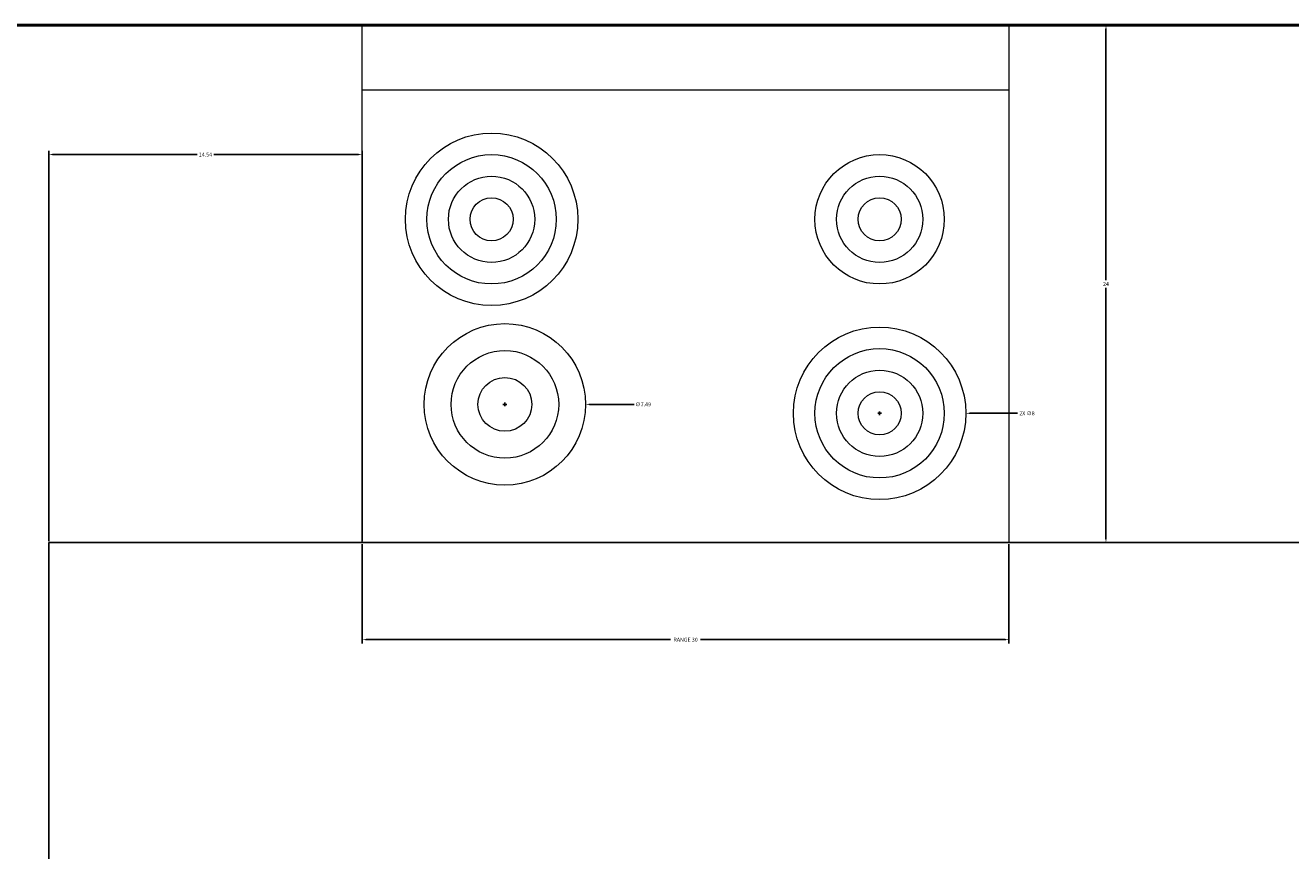
# Model space of a CAD drawing. Units: inches. Extents: x 2621 to 2849, y 2066 to 2463.
# Tile 10 of 28: x 2671 to 2729, y 2277 to 2315. Entities that reach past the tile are written whole.
import ezdxf

# ---------------------------------------------------------------- set-up
doc = ezdxf.new("R2010")
doc.units = ezdxf.units.IN
for name, color, linetype, lineweight in [('A-ANNO-DIMS', 2, 'Continuous', 18), ('A-EQPM', 8, 'Continuous', 18), ('A-FLOR-CASE', 9, 'Continuous', 25), ('A-WALL', 7, 'Continuous', 50)]:
    doc.layers.add(name, color=color, linetype=linetype, lineweight=lineweight)
doc.styles.get("Standard").update_dxf_attribs({"font": 'arial.ttf'})
doc.dimstyles.get("Standard").update_dxf_attribs({"dimtxt": 0.18, "dimasz": 0.18, "dimexe": 0.18, "dimexo": 0.0625, "dimgap": 0.09, "dimtad": 0, "dimtih": 1, "dimtoh": 1, "dimdec": 4, "dimzin": 0, "dimdsep": 46, "dimtxsty": 'Standard', "dimcen": 0.09, "dimadec": 0, "dimazin": 0, "dimtfac": 1, "dimtdec": 4, "dimtofl": 0, "dimtmove": 0, "dimatfit": 3, "dimfxl": 1, "dimtolj": 1, "dimtzin": 0, "dimarcsym": 0})

# ---------------------------------------------------------------- blocks, each defined once
blk = doc.blocks.new('Range-Oven - 30 in top')
blk.add_line((0, -3), (30, -3))
blk.add_lwpolyline([(0, -24), (0, 0), (30, 0), (30, -24)], close=True)
for centre, radius in [((6, -9), 4), ((6, -9), 3), ((24, -9), 3), ((6, -9), 2), ((24, -9), 2), ((6, -9), 1), ((24, -9), 1), ((6.618, -17.584), 3.745), ((24, -18), 4), ((6.618, -17.584), 2.496), ((24, -18), 3), ((6.618, -17.584), 1.248), ((24, -18), 2), ((24, -18), 1)]:
    blk.add_circle(centre, radius)
blk = doc.blocks.new('*D21')
at = {"layer": 'A-ANNO-DIMS', "color": 0, "lineweight": -2, "transparency": 16777216}
for p, q in [((2686.41, 2291.312), (2686.41, 2286.695)), ((2716.41, 2291.312), (2716.41, 2286.695)), ((2686.59, 2286.875), (2700.714, 2286.875)), ((2716.23, 2286.875), (2702.106, 2286.875))]:
    blk.add_line(p, q, dxfattribs=at)
at = {"layer": 'A-ANNO-DIMS', "color": 0, "transparency": 16777216}
for points in [[(2686.59, 2286.905), (2686.59, 2286.845), (2686.41, 2286.875)], [(2716.23, 2286.905), (2716.23, 2286.845), (2716.41, 2286.875)]]:
    blk.add_solid(points, dxfattribs=at)
at = {"layer": 'Defpoints', "color": 0, "transparency": 16777216}
for p in [(2686.41, 2291.375), (2716.41, 2291.375), (2716.41, 2286.875)]:
    blk.add_point(p, dxfattribs=at)
at = {"layer": 'A-ANNO-DIMS', "color": 0, "transparency": 16777216, "insert": (2701.41, 2286.875), "char_height": 0.18, "attachment_point": 5}
blk.add_mtext('\\A1;RANGE 30', dxfattribs=at)
blk = doc.blocks.new('*D22')
at = {"layer": 'A-ANNO-DIMS', "color": 0, "lineweight": -2, "transparency": 16777216}
for p, q in [((2716.473, 2315.375), (2721.09, 2315.375)), ((2720.91, 2315.195), (2720.91, 2303.555)), ((2720.91, 2291.555), (2720.91, 2303.194)), ((2716.473, 2291.375), (2721.09, 2291.375))]:
    blk.add_line(p, q, dxfattribs=at)
at = {"layer": 'A-ANNO-DIMS', "color": 0, "transparency": 16777216}
for points in [[(2720.88, 2315.195), (2720.94, 2315.195), (2720.91, 2315.375)], [(2720.88, 2291.555), (2720.94, 2291.555), (2720.91, 2291.375)]]:
    blk.add_solid(points, dxfattribs=at)
at = {"layer": 'Defpoints', "color": 0, "transparency": 16777216}
for p in [(2716.41, 2315.375), (2720.91, 2315.375), (2716.41, 2291.375)]:
    blk.add_point(p, dxfattribs=at)
at = {"layer": 'A-ANNO-DIMS', "color": 0, "transparency": 16777216, "insert": (2720.91, 2303.375), "char_height": 0.18, "attachment_point": 5}
blk.add_mtext('\\A1;24', dxfattribs=at)
blk = doc.blocks.new('*D66')
at = {"layer": 'A-ANNO-DIMS', "color": 0, "lineweight": -2, "transparency": 16777216}
for p, q in [((2671.87, 2291.437), (2671.87, 2309.558)), ((2672.05, 2309.378), (2678.755, 2309.378)), ((2686.23, 2309.378), (2679.525, 2309.378)), ((2686.41, 2291.437), (2686.41, 2309.558))]:
    blk.add_line(p, q, dxfattribs=at)
at = {"layer": 'A-ANNO-DIMS', "color": 0, "transparency": 16777216}
for points in [[(2672.05, 2309.408), (2672.05, 2309.348), (2671.87, 2309.378)], [(2686.23, 2309.408), (2686.23, 2309.348), (2686.41, 2309.378)]]:
    blk.add_solid(points, dxfattribs=at)
at = {"layer": 'Defpoints', "color": 0, "transparency": 16777216}
for p in [(2686.41, 2309.378), (2671.87, 2291.375), (2686.41, 2291.375)]:
    blk.add_point(p, dxfattribs=at)
at = {"layer": 'A-ANNO-DIMS', "color": 0, "transparency": 16777216, "insert": (2679.14, 2309.378), "char_height": 0.18, "attachment_point": 5}
blk.add_mtext('\\A1;14.54', dxfattribs=at)
blk = doc.blocks.new('*D73')
at = {"layer": 'A-ANNO-DIMS', "color": 0, "lineweight": -2, "transparency": 16777216}
for p, q in [((2710.41, 2297.285), (2710.41, 2297.465)), ((2710.32, 2297.375), (2710.5, 2297.375)), ((2716.81, 2297.375), (2714.59, 2297.375))]:
    blk.add_line(p, q, dxfattribs=at)
at = {"layer": 'A-ANNO-DIMS', "color": 0, "transparency": 16777216}
blk.add_solid([(2714.59, 2297.405), (2714.59, 2297.345), (2714.41, 2297.375)], dxfattribs=at)
at = {"layer": 'Defpoints', "color": 0, "transparency": 16777216}
for p in [(2706.41, 2297.374), (2714.41, 2297.375)]:
    blk.add_point(p, dxfattribs=at)
at = {"layer": 'A-ANNO-DIMS', "color": 0, "transparency": 16777216, "insert": (2717.247, 2297.375), "char_height": 0.18, "attachment_point": 5}
blk.add_mtext('\\A1;2X ∅8', dxfattribs=at)
blk = doc.blocks.new('*D75')
at = {"layer": 'A-ANNO-DIMS', "color": 0, "lineweight": -2, "transparency": 16777216}
for p, q in [((2692.938, 2297.791), (2693.118, 2297.791)), ((2693.028, 2297.701), (2693.028, 2297.881)), ((2699.019, 2297.791), (2696.953, 2297.791))]:
    blk.add_line(p, q, dxfattribs=at)
at = {"layer": 'A-ANNO-DIMS', "color": 0, "transparency": 16777216}
blk.add_solid([(2696.953, 2297.821), (2696.953, 2297.761), (2696.773, 2297.791)], dxfattribs=at)
at = {"layer": 'Defpoints', "color": 0, "transparency": 16777216}
for p in [(2689.283, 2297.79), (2696.773, 2297.791)]:
    blk.add_point(p, dxfattribs=at)
at = {"layer": 'A-ANNO-DIMS', "color": 0, "transparency": 16777216, "insert": (2699.441, 2297.791), "char_height": 0.18, "attachment_point": 5}
blk.add_mtext('\\A1;∅7.49', dxfattribs=at)

msp = doc.modelspace()

# ---------------------------------------------------------------- linework, layer by layer
at = {"layer": 'A-FLOR-CASE'}
for p, q in [((2671.8701, 2291.3746), (2763.8701, 2291.3746)), ((2671.8701, 2199.3746), (2671.8701, 2291.3746))]:
    msp.add_line(p, q, dxfattribs=at)
at = {"layer": 'A-WALL'}
msp.add_line((2647.8701, 2315.3746), (2763.8701, 2315.3746), dxfattribs=at)

# ---------------------------------------------------------------- block references
at = {"layer": 'A-EQPM'}
msp.add_blockref('Range-Oven - 30 in top', (2686.4102, 2315.3746), dxfattribs=at)

# ---------------------------------------------------------------- dimensions: what is measured, and where the dimension line sits
at = {"layer": 'A-ANNO-DIMS'}
for base, p1, p2, angle, override, picture, middle in [((2720.9102, 2315.3746), (2716.4102, 2291.3746), (2716.4102, 2315.3746), 90, {"dimdec": 0, "dimlfac": 1, "dimrnd": 0, "dimzin": 0, "dimdsep": 46, "dimlunit": 2}, '*D22', (2720.9102, 2303.3746)), ((2686.4102, 2309.3781), (2671.8701, 2291.3746), (2686.4102, 2291.3746), 0.000016, {"dimdec": 2, "dimlfac": 1, "dimrnd": 0, "dimzin": 0, "dimdsep": 46, "dimlunit": 2}, '*D66', (2679.1401, 2309.3781))]:
    dim = msp.add_linear_dim(base=base, p1=p1, p2=p2, angle=angle, dimstyle='Standard', override=override, dxfattribs=at)
    dim.commit()
    dim.dimension.update_dxf_attribs({"geometry": picture, "text_midpoint": middle})
dim = msp.add_diameter_dim_2p(p1=(2689.2832, 2297.7902), p2=(2696.7726, 2297.791), dimstyle='Standard', override={"dimdec": 2, "dimlfac": 1, "dimrnd": 0, "dimzin": 0, "dimdsep": 46, "dimlunit": 2}, dxfattribs=at)
dim.commit()
dim.dimension.update_dxf_attribs({"geometry": '*D75', "text_midpoint": (2699.0195, 2297.7913), "dimtype": 163})
dim = msp.add_diameter_dim_2p(p1=(2706.4102, 2297.3742), p2=(2714.4102, 2297.375), text='2X <>', dimstyle='Standard', override={"dimdec": 0, "dimlfac": 1, "dimrnd": 0, "dimzin": 0, "dimdsep": 46, "dimlunit": 2}, dxfattribs=at)
dim.commit()
dim.dimension.update_dxf_attribs({"geometry": '*D73', "text_midpoint": (2716.8102, 2297.3752), "dimtype": 163})
dim = msp.add_linear_dim(base=(2716.4102, 2286.8746), p1=(2686.4102, 2291.3746), p2=(2716.4102, 2291.3746), text='RANGE <>', dimstyle='Standard', override={"dimdec": 0, "dimlfac": 1, "dimrnd": 0, "dimzin": 0, "dimdsep": 46, "dimlunit": 2}, dxfattribs=at)
dim.commit()
dim.dimension.update_dxf_attribs({"geometry": '*D21', "text_midpoint": (2701.4102, 2286.8746)})

doc.saveas('drawing.dxf')
